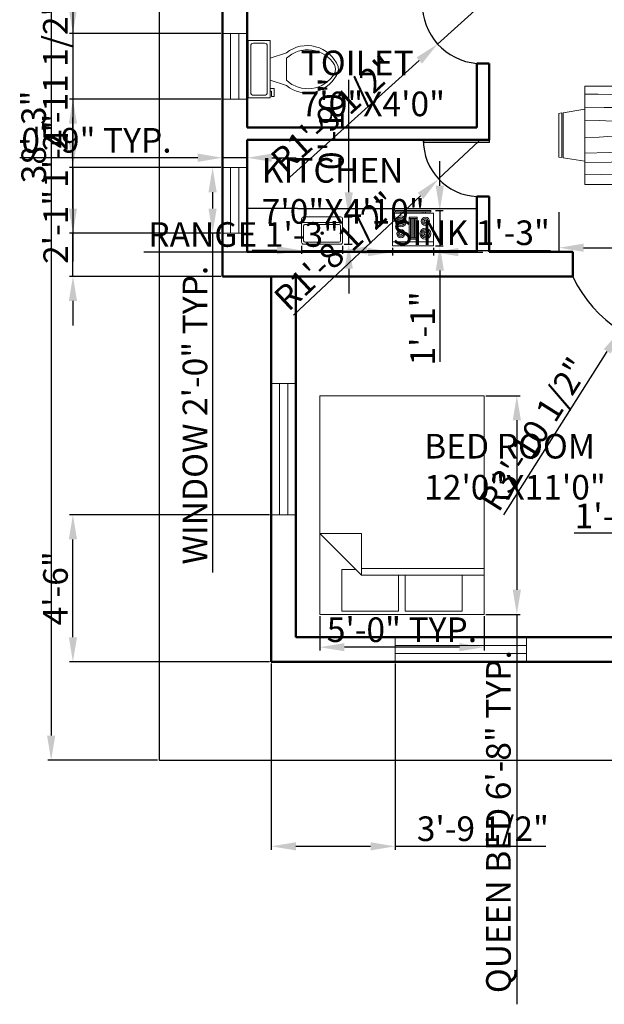
# Model space of a CAD drawing. Units: inches. Extents: x 2059616 to 2060276, y 889994 to 890582.
# Tile 1 of 4: x 2059616 to 2059830, y 889994 to 890354. Entities that reach past the tile are written whole.
import ezdxf

# ---------------------------------------------------------------- set-up
doc = ezdxf.new("R2010")
doc.units = ezdxf.units.IN
for name, color, linetype, lineweight in [('A-ANNO-DIMS', 2, 'Continuous', 18), ('A-AREA-IDEN', 7, 'Continuous', 25), ('A-DOOR', 3, 'Continuous', 25), ('A-EQPM', 9, 'Continuous', 18), ('A-FLOR-CASE', 9, 'Continuous', 25), ('A-FLOR-FIXT', 9, 'Continuous', 18), ('A-FURN', 8, 'Continuous', 18), ('A-GLAZ', 4, 'Continuous', 18), ('A-WALL', 7, 'Continuous', 50), ('C-PROP', 7, 'Continuous', 25)]:
    doc.layers.add(name, color=color, linetype=linetype, lineweight=lineweight)
doc.styles.get("Standard").update_dxf_attribs({"font": 'arial.ttf'})
doc.dimstyles.new('ISO-25', dxfattribs={"dimtxt": 9, "dimasz": 9, "dimexe": 1.25, "dimexo": 0.625, "dimtad": 1, "dimdec": 1, "dimrnd": 9, "dimlunit": 3, "dimtxsty": 'Standard', "dimcen": 2.5, "dimadec": 0, "dimazin": 0, "dimtfac": 1, "dimtdec": 1, "dimtmove": 0, "dimatfit": 3, "dimfxl": 1, "dimarcsym": 0})

# ---------------------------------------------------------------- blocks, each defined once
blk = doc.blocks.new('*D2')
at = {"layer": 'A-ANNO-DIMS', "color": 0, "lineweight": -2, "transparency": 16777216}
for p, q in [((2059666.14, 890538.85), (2059626.05, 890538.85)), ((2059627.3, 890529.85), (2059627.3, 890091.85)), ((2059666.14, 890082.85), (2059626.05, 890082.85))]:
    blk.add_line(p, q, dxfattribs=at)
at = {"layer": 'A-ANNO-DIMS', "color": 0, "transparency": 16777216}
for points in [[(2059625.8, 890529.85), (2059628.8, 890529.85), (2059627.3, 890538.85)], [(2059625.8, 890091.85), (2059628.8, 890091.85), (2059627.3, 890082.85)]]:
    blk.add_solid(points, dxfattribs=at)
at = {"layer": 'Defpoints', "color": 0, "transparency": 16777216}
for p in [(2059666.76, 890538.85), (2059627.3, 890082.85), (2059666.76, 890082.85)]:
    blk.add_point(p, dxfattribs=at)
at = {"layer": 'A-ANNO-DIMS', "color": 0, "transparency": 16777216, "insert": (2059622.08, 890310.85), "char_height": 9, "attachment_point": 5, "rotation": 90}
blk.add_mtext('38\'-3"', dxfattribs=at)
blk = doc.blocks.new('Bed - Queen')
for p, q in [((0, -80.00003), (0, 0)), ((0, 0), (59.99999, 0)), ((59.99999, 0), (59.99999, -80.00003)), ((7.99999, -1.2), (28.79998, -1.2)), ((7.99999, -14.4), (7.99999, -1.2)), ((28.79998, -1.2), (28.79998, -14.4)), ((31.19999, -1.2), (51.99999, -1.2)), ((31.19999, -14.4), (31.19999, -1.2)), ((51.99999, -1.2), (51.99999, -16.4)), ((0, -14.4), (44.8, -14.4)), ((59.99999, -29.6), (44.8, -14.4)), ((44.8, -14.4), (44.8, -29.6)), ((44.8, -16.8), (0, -16.8)), ((51.99999, -16.4), (46.79936, -16.4)), ((44.8, -29.6), (59.99999, -29.6)), ((59.99999, -80.00003), (0, -80.00003))]:
    blk.add_line(p, q)
blk = doc.blocks.new('Toilet - top')
for p, q in [((9.5, -6), (9.5, -2)), ((-10, -8.5), (-8, -8.5)), ((-10, -9.5), (-10, -8.5)), ((-7, -9.5), (-10, -9.5)), ((-8, -8.5), (-8, -8)), ((-7, -8), (-7, -9.5)), ((-4, -8), (-6, -14)), ((4, -8), (6, -14)), ((4, -14), (-4, -14))]:
    blk.add_line(p, q)
blk.add_lwpolyline([(10.5, -8), (10.5, 0), (-10.5, 0), (-10.5, -8)], close=True)
for points in [[(-9.5, -2), (-9.5, -6)], [(8.5, -1), (-8.5, -1)], [(-8.5, -7), (8.5, -7)]]:
    blk.add_lwpolyline(points)
for centre, radius, start, end in [((-8.62, -1.88), 0.884, 81.8699, 188.1301), ((8.62, -1.88), 0.884, 351.8699, 98.1301), ((-8.62, -6.12), 0.884, 171.8699, 278.1301), ((8.62, -6.12), 0.884, 261.8699, 8.1301), ((3.52, -21.58), 12.17, 141.4691, 247.9714), ((4.2, -21.82), 11.33, 136.3677, 238.9468), ((-3.52, -21.58), 12.17, 292.0284, 38.5307), ((-4.2, -21.82), 11.33, 301.053, 43.6321), ((0, -27.88), 4, 245.7318, 294.2682), ((0, -29), 4, 254.8605, 285.1395)]:
    blk.add_arc(centre, radius, start, end)
blk = doc.blocks.new('Range-Oven - 30 in top')
for p, q in [((0, -3), (30, -3)), ((12, -6), (18, -6)), ((13, -20), (13, -6)), ((14, -6), (14, -20)), ((15, -20), (15, -6)), ((16, -6), (16, -20)), ((17, -20), (17, -6)), ((18, -20), (12, -20)), ((6, -24), (6, -25)), ((8, -25), (8, -24)), ((22, -25), (22, -24)), ((24, -24), (24, -25))]:
    blk.add_line(p, q)
for points in [[(0, -24), (0, 0), (30, 0), (30, -24)], [(12, -21), (12, -5), (18, -5), (18, -21)], [(2, -26), (2, -25), (28, -25), (28, -26)]]:
    blk.add_lwpolyline(points, close=True)
for centre, radius in [((6, -9), 4), ((6, -9), 3), ((6, -9), 2), ((24, -9), 3), ((24, -9), 2), ((6, -9), 1), ((24, -18), 4), ((24, -9), 1), ((6, -18), 3), ((6, -18), 2), ((6, -18), 1), ((24, -18), 3), ((24, -18), 2), ((24, -18), 1)]:
    blk.add_circle(centre, radius)
blk = doc.blocks.new('Sink-single - 30 in top')
blk.add_line((-15, -3.999996), (15, -3.999996))
for points in [[(-13.5, 0), (13.5, 0)], [(-15, -18.499996), (-15, -1.5)], [(-13.5, -17.499996), (-13.5, -6.499996)], [(-12.5, -5.499996), (12.5, -5.499996)], [(13.5, -6.499996), (13.5, -17.499996)], [(15, -1.5), (15, -18.499996)], [(13.5, -19.999996), (-13.5, -19.999996)], [(12.5, -18.499996), (-12.5, -18.499996)]]:
    blk.add_lwpolyline(points)
for radius in [1, 0.5]:
    blk.add_circle((0, -11.999996), radius)
for centre, radius, start, end in [((-13.5, -1.5), 1.5, 90, 180), ((-12.5, -6.499996), 1, 90, 180), ((12.5, -6.499996), 1, 0, 90), ((13.5, -1.5), 1.5, 0, 90), ((-13.5, -18.499996), 1.5, 180, 270), ((-12.5, -17.499996), 1, 180, 270), ((12.5, -17.499996), 1, 270, 0), ((13.5, -18.499996), 1.5, 270, 0)]:
    blk.add_arc(centre, radius, start, end)
blk = doc.blocks.new('Dining Set - 36 x 72 in.')
for p, q in [((-22.2343, 26.00059), (-23.4847, 17.99762)), ((-22.2304, 26), (-5.7608, 26)), ((-22, 27.5), (-22.1562, 26.50042)), ((-5.8416, 26.5), (-22.1534, 26.5)), ((-22, 27.5), (-6, 27.5)), ((-5.8437, 26.49966), (-6, 27.5)), ((-4.5152, 17.99762), (-5.7655, 25.99926)), ((5.7657, 26.00059), (4.5153, 17.99762)), ((5.7696, 26), (22.2392, 26)), ((6, 27.5), (5.8438, 26.50042)), ((22.1584, 26.5), (5.8466, 26.5)), ((6, 27.5), (22, 27.5)), ((22.1563, 26.49966), (22, 27.5)), ((23.4848, 17.99762), (22.2345, 25.99926)), ((36, 18), (-36, 18)), ((-36, 18), (-36, -18)), ((36, -18), (36, 18)), ((-45.5, 8), (-44.5004, 8.15617)), ((-45.5, 8), (-45.5, -8)), ((-44.5, -8.15843), (-44.5, 8.15338)), ((-44.0006, 8.23428), (-35.9976, 9.48474)), ((-44, 8.23041), (-44, -8.23915)), ((44.0006, 8.23428), (35.9976, 9.48474)), ((44, 8.23041), (44, -8.23915)), ((44.5, -8.15843), (44.5, 8.15338)), ((45.5, 8), (44.5005, 8.15617)), ((45.5, 8), (45.5, -8)), ((-44.4997, -8.15631), (-45.5, -8)), ((-35.9976, -9.48476), (-43.9993, -8.2345)), ((35.9976, -9.48476), (43.9993, -8.2345)), ((44.4997, -8.15631), (45.5, -8)), ((-36, -18), (36, -18)), ((-22.2343, -26.0006), (-23.4847, -17.99762)), ((-4.5152, -17.99762), (-5.7655, -25.99928)), ((5.7657, -26.0006), (4.5153, -17.99762)), ((23.4848, -17.99762), (22.2345, -25.99928)), ((-22.2304, -26), (-5.7608, -26)), ((-22, -27.5), (-22.1562, -26.50044)), ((-5.8416, -26.5), (-22.1534, -26.5)), ((-22, -27.5), (-6, -27.5)), ((-5.8437, -26.49967), (-6, -27.5)), ((5.7696, -26), (22.2392, -26)), ((6, -27.5), (5.8438, -26.50044)), ((22.1584, -26.5), (5.8466, -26.5)), ((6, -27.5), (22, -27.5)), ((22.1563, -26.49967), (22, -27.5))]:
    blk.add_line(p, q)
for points in [[(-36, 15), (-31.1772, 14.97754), (-26.8079, 14.91406), (-22.8538, 14.81543), (-19.276, 14.6875), (-16.0362, 14.53613), (-13.0957, 14.36718), (-10.4159, 14.18652), (-7.9583, 14), (-5.6904, 13.81315), (-3.6035, 13.63021), (-1.6954, 13.45508), (0.0365, 13.29166), (1.5945, 13.14388), (2.9811, 13.01562), (4.1988, 12.9108), (5.25, 12.83333), (6.1393, 12.78613), (6.8802, 12.76823), (7.4883, 12.77767), (7.9792, 12.8125), (8.3685, 12.87077), (8.6719, 12.95052), (8.9049, 13.0498), (9.0833, 13.16666), (9.2205, 13.29899), (9.3216, 13.44401), (9.3895, 13.59879), (9.4271, 13.76041), (9.4373, 13.92594), (9.4232, 14.09245), (9.3875, 14.257), (9.3333, 14.41666), (9.2638, 14.56917), (9.1836, 14.71484), (9.0975, 14.85465), (9.0104, 14.98958), (8.9272, 15.1206), (8.8529, 15.2487), (8.7922, 15.37483), (8.75, 15.5), (8.7305, 15.62467), (8.7344, 15.74739), (8.7617, 15.86621), (8.8125, 15.97916), (8.8867, 16.08431), (8.9844, 16.17968), (9.1055, 16.26334), (9.25, 16.33333), (9.4189, 16.38802), (9.6172, 16.42708), (9.8506, 16.45052), (10.125, 16.45833), (10.4463, 16.45052), (10.8203, 16.42708), (11.2529, 16.38802), (11.75, 16.33333), (12.3184, 16.26318), (12.9694, 16.17838), (13.7151, 16.07991), (14.5677, 15.96875), (15.5395, 15.84586), (16.6426, 15.71224), (17.8893, 15.56884), (19.2917, 15.41666), (20.859, 15.25667), (22.5879, 15.08984), (24.4721, 14.91715), (26.5052, 14.73958), (28.6809, 14.5581), (30.9929, 14.3737), (33.4347, 14.18733), (36, 14)], [(-36, 10), (-28.9766, 10.14274), (-23.1725, 10.20442), (-18.4241, 10.19775), (-14.5677, 10.13541), (-11.4399, 10.03011), (-8.877, 9.89453), (-6.7154, 9.74137), (-4.7917, 9.58333), (-2.9698, 9.43082), (-1.2246, 9.28515), (0.4415, 9.14534), (2.026, 9.01041), (3.5266, 8.87939), (4.9408, 8.7513), (6.266, 8.62516), (7.5, 8.5), (8.6411, 8.37549), (9.6914, 8.2539), (10.6538, 8.13818), (11.5312, 8.03125), (12.3267, 7.93603), (13.043, 7.85547), (13.6831, 7.79248), (14.25, 7.75), (14.7471, 7.7303), (15.1797, 7.73307), (15.5537, 7.75732), (15.875, 7.80208), (16.1494, 7.86637), (16.3828, 7.94922), (16.5811, 8.04964), (16.75, 8.16666), (16.8944, 8.29915), (17.0143, 8.44531), (17.1089, 8.60319), (17.1771, 8.77083), (17.218, 8.94629), (17.2305, 9.1276), (17.2137, 9.31282), (17.1667, 9.5), (17.0895, 9.6875), (16.987, 9.875), (16.8649, 10.0625), (16.7292, 10.25), (16.5856, 10.4375), (16.4401, 10.625), (16.2985, 10.8125), (16.1667, 11), (16.05, 11.18733), (15.9518, 11.3737), (15.8752, 11.5581), (15.8229, 11.73958), (15.798, 11.91715), (15.8034, 12.08984), (15.842, 12.25667), (15.9167, 12.41666), (16.0295, 12.56836), (16.1784, 12.70833), (16.3605, 12.83268), (16.5729, 12.9375), (16.8127, 13.01888), (17.0768, 13.07291), (17.3625, 13.0957), (17.6667, 13.08333), (17.9894, 13.03312), (18.3418, 12.94726), (18.7382, 12.82918), (19.1927, 12.68229), (19.7195, 12.51001), (20.3327, 12.31575), (21.0465, 12.10294), (21.875, 11.875), (22.8357, 11.63354), (23.959, 11.37304), (25.2786, 11.08618), (26.8282, 10.76562), (28.6414, 10.40405), (30.752, 9.99414), (33.1936, 9.52856), (36, 9)], [(-36, 5.5), (-30.7157, 5.3348), (-26.069, 5.20963), (-21.9946, 5.11767), (-18.4271, 5.05208), (-15.3009, 5.00602), (-12.5508, 4.97265), (-10.1112, 4.94515), (-7.9167, 4.91666), (-5.909, 4.88167), (-4.0586, 4.83984), (-2.3429, 4.79215), (-0.7396, 4.73958), (0.7739, 4.6831), (2.22, 4.6237), (3.6213, 4.56233), (5, 4.5), (6.373, 4.43782), (7.7344, 4.3776), (9.0723, 4.32129), (10.375, 4.27083), (11.6309, 4.22819), (12.8281, 4.19531), (13.9551, 4.17415), (15, 4.16666), (15.954, 4.17448), (16.819, 4.19791), (17.6001, 4.23698), (18.3021, 4.29166), (18.9299, 4.36198), (19.4883, 4.44791), (19.9823, 4.54948), (20.4167, 4.66666), (20.7969, 4.79899), (21.1302, 4.94401), (21.4245, 5.09879), (21.6875, 5.26041), (21.9271, 5.42594), (22.1511, 5.59245), (22.3672, 5.757), (22.5834, 5.91666), (22.8065, 6.06868), (23.0404, 6.21093), (23.2879, 6.34147), (23.5521, 6.45833), (23.8358, 6.55957), (24.142, 6.64323), (24.4735, 6.70735), (24.8334, 6.75), (25.2235, 6.76969), (25.642, 6.76692), (26.0858, 6.74267), (26.5521, 6.69791), (27.0379, 6.63362), (27.5404, 6.55078), (28.0565, 6.45036), (28.5834, 6.33333), (29.1242, 6.19987), (29.7071, 6.04687), (30.3661, 5.87044), (31.1354, 5.66666), (32.0493, 5.43164), (33.142, 5.16146), (34.4475, 4.85221), (36, 4.5)], [(-36, -1), (-30.7915, -0.6591), (-26.0195, -0.38216), (-21.6519, -0.16284), (-17.6563, 0.00521), (-14.0005, 0.12833), (-10.6523, 0.21289), (-7.5796, 0.26522), (-4.75, 0.29166), (-2.134, 0.29793), (0.2878, 0.28711), (2.5317, 0.26163), (4.6146, 0.22396), (6.5529, 0.17651), (8.3633, 0.12174), (10.0623, 0.06209), (11.6667, 0), (13.1899, -0.06201), (14.6341, -0.1211), (15.9982, -0.17432), (17.2813, -0.21875), (18.4823, -0.25147), (19.6003, -0.26953), (20.6343, -0.27002), (21.5834, -0.25), (22.4481, -0.20768), (23.2357, -0.14584), (23.9549, -0.06836), (24.6146, 0.02083), (25.2235, 0.11784), (25.7904, 0.21875), (26.3241, 0.31966), (26.8334, 0.41666), (27.3265, 0.50618), (27.8099, 0.58593), (28.2894, 0.65397), (28.7709, 0.70833), (29.2601, 0.74707), (29.763, 0.76823), (30.2855, 0.76985), (30.8334, 0.75), (31.4088, 0.70784), (31.9994, 0.64713), (32.589, 0.57275), (33.1615, 0.48958), (33.7008, 0.4025), (34.1908, 0.3164), (34.6153, 0.23616), (34.9584, 0.16666), (35.2099, 0.11165), (35.3848, 0.07031), (35.504, 0.04069), (35.5886, 0.02083), (35.6594, 0.00879), (35.7377, 0.0026), (35.8442, 0.00032), (36, 0)], [(-36, -6.5), (-27.1843, -6.31267), (-20.084, -6.1263), (-14.469, -5.9419), (-10.1094, -5.76042), (-6.7752, -5.58285), (-4.2363, -5.41016), (-2.2629, -5.24333), (-0.625, -5.08334), (0.8708, -4.93099), (2.2715, -4.78646), (3.5872, -4.64974), (4.8281, -4.52084), (6.0046, -4.39974), (7.127, -4.28646), (8.2053, -4.18099), (9.25, -4.08334), (10.2705, -3.99382), (11.2734, -3.91407), (12.2647, -3.84603), (13.25, -3.79167), (14.2354, -3.75293), (15.2266, -3.73177), (16.2295, -3.73015), (17.25, -3.75), (18.2912, -3.79248), (19.3451, -3.85547), (20.4009, -3.93604), (21.4479, -4.03125), (22.4754, -4.13819), (23.4727, -4.25391), (24.4289, -4.37549), (25.3334, -4.5), (26.1785, -4.62492), (26.9694, -4.74935), (27.7145, -4.87281), (28.4219, -4.99479), (29.1, -5.11483), (29.7572, -5.23242), (30.4016, -5.34709), (31.0417, -5.45834), (31.6837, -5.56437), (32.3262, -5.65821), (32.9658, -5.73153), (33.599, -5.77604), (34.2224, -5.78345), (34.8327, -5.74545), (35.4264, -5.65373), (36, -5.5)], [(-36, -10), (-26.4022, -9.81299), (-18.4675, -9.62891), (-11.9839, -9.45069), (-6.7396, -9.28125), (-2.5226, -9.12354), (0.8789, -8.98047), (3.6769, -8.85498), (6.0833, -8.75), (8.2767, -8.66765), (10.3021, -8.60677), (12.1712, -8.56543), (13.8958, -8.54167), (15.4876, -8.53353), (16.9583, -8.53907), (18.3197, -8.55632), (19.5834, -8.58334), (20.7616, -8.61841), (21.8685, -8.66081), (22.9188, -8.71004), (23.9271, -8.76563), (24.9081, -8.82707), (25.8763, -8.89388), (26.8465, -8.96558), (27.8334, -9.04167), (28.8474, -9.12118), (29.8828, -9.20117), (30.93, -9.27824), (31.9792, -9.34896), (33.0205, -9.40991), (34.0443, -9.45768), (35.0407, -9.48885), (36, -9.5)], [(-36, -14.5), (-30.0881, -14.33513), (-25.0332, -14.21224), (-20.7312, -14.12647), (-17.0781, -14.07292), (-13.97, -14.04671), (-11.3027, -14.04297), (-8.9724, -14.05681), (-6.875, -14.08334), (-4.9224, -14.11833), (-3.0905, -14.16016), (-1.3709, -14.20785), (0.2448, -14.26042), (1.7647, -14.3169), (3.1973, -14.3763), (4.5507, -14.43767), (5.8333, -14.5), (7.0554, -14.5621), (8.235, -14.62175), (9.3922, -14.67652), (10.5469, -14.72396), (11.7192, -14.76164), (12.929, -14.78711), (14.1965, -14.79794), (15.5417, -14.79167), (16.9933, -14.76424), (18.6152, -14.70508), (20.4804, -14.60197), (22.6615, -14.44271), (25.2312, -14.21509), (28.2624, -13.9069), (31.8277, -13.50594), (36, -13)]]:
    blk.add_lwpolyline(points)
blk = doc.blocks.new('WIN-48IN')
for p, q in [((0, 9), (0, 0)), ((48, 9), (48, 0)), ((48, 6), (0, 6)), ((48, 3), (0, 3))]:
    blk.add_line(p, q)
blk = doc.blocks.new('WIN-24IN')
for p, q in [((0, 24), (9, 24)), ((3, 24), (3, 0)), ((6, 24), (6, 0)), ((0, 0), (9, 0))]:
    blk.add_line(p, q)
blk = doc.blocks.new('*D18')
at = {"layer": 'A-ANNO-DIMS', "color": 0, "lineweight": -2, "transparency": 16777216}
for p, q in [((2059689.29, 890299.64), (2059685.06, 890299.64)), ((2059686.31, 890290.64), (2059686.31, 890284.64)), ((2059689.29, 890275.64), (2059685.06, 890275.64)), ((2059686.31, 890275.64), (2059686.31, 890151.5))]:
    blk.add_line(p, q, dxfattribs=at)
at = {"layer": 'A-ANNO-DIMS', "color": 0, "transparency": 16777216}
for points in [[(2059684.81, 890290.64), (2059687.81, 890290.64), (2059686.31, 890299.64)], [(2059684.81, 890284.64), (2059687.81, 890284.64), (2059686.31, 890275.64)]]:
    blk.add_solid(points, dxfattribs=at)
at = {"layer": 'Defpoints', "color": 0, "transparency": 16777216}
for p in [(2059689.91, 890299.64), (2059686.31, 890275.64), (2059689.91, 890275.64)]:
    blk.add_point(p, dxfattribs=at)
at = {"layer": 'A-ANNO-DIMS', "color": 0, "transparency": 16777216, "insert": (2059681.03, 890209.07), "char_height": 9, "attachment_point": 5, "rotation": 90}
blk.add_mtext('WINDOW 2\'-0" TYP.', dxfattribs=at)
blk = doc.blocks.new('*D19')
at = {"layer": 'A-ANNO-DIMS', "color": 0, "lineweight": -2, "transparency": 16777216}
for p, q in [((2059680.91, 890303.24), (2059615.81, 890303.24)), ((2059689.91, 890300.26), (2059689.91, 890304.49)), ((2059698.91, 890303.24), (2059689.91, 890303.24)), ((2059698.91, 890300.26), (2059698.91, 890304.49)), ((2059707.91, 890303.24), (2059716.91, 890303.24))]:
    blk.add_line(p, q, dxfattribs=at)
at = {"layer": 'A-ANNO-DIMS', "color": 0, "transparency": 16777216}
for points in [[(2059680.91, 890304.74), (2059680.91, 890301.74), (2059689.91, 890303.24)], [(2059707.91, 890304.74), (2059707.91, 890301.74), (2059698.91, 890303.24)]]:
    blk.add_solid(points, dxfattribs=at)
at = {"layer": 'Defpoints', "color": 0, "transparency": 16777216}
for p in [(2059689.91, 890303.24), (2059689.91, 890299.64), (2059698.91, 890299.64)]:
    blk.add_point(p, dxfattribs=at)
at = {"layer": 'A-ANNO-DIMS', "color": 0, "transparency": 16777216, "insert": (2059643.86, 890308.46), "char_height": 9, "attachment_point": 5}
blk.add_mtext('0\'-9" TYP.', dxfattribs=at)
blk = doc.blocks.new('*D22')
at = {"layer": 'A-ANNO-DIMS', "color": 0, "lineweight": -2, "transparency": 16777216}
for p, q in [((2059786.15, 890216.2), (2059798.78, 890216.2)), ((2059797.53, 890207.2), (2059797.53, 890145.2)), ((2059786.15, 890136.2), (2059798.78, 890136.2)), ((2059797.53, 890136.2), (2059797.53, 889993.56))]:
    blk.add_line(p, q, dxfattribs=at)
at = {"layer": 'A-ANNO-DIMS', "color": 0, "transparency": 16777216}
for points in [[(2059796.03, 890207.2), (2059799.03, 890207.2), (2059797.53, 890216.2)], [(2059796.03, 890145.2), (2059799.03, 890145.2), (2059797.53, 890136.2)]]:
    blk.add_solid(points, dxfattribs=at)
at = {"layer": 'Defpoints', "color": 0, "transparency": 16777216}
for p in [(2059785.53, 890216.2), (2059785.53, 890136.2), (2059797.53, 890136.2)]:
    blk.add_point(p, dxfattribs=at)
at = {"layer": 'A-ANNO-DIMS', "color": 0, "transparency": 16777216, "insert": (2059791.97, 890060.38), "char_height": 9, "attachment_point": 5, "rotation": 90}
blk.add_mtext('QUEEN BED 6\'-8" TYP.', dxfattribs=at)
blk = doc.blocks.new('*D23')
at = {"layer": 'A-ANNO-DIMS', "color": 0, "lineweight": -2, "transparency": 16777216}
for p, q in [((2059725.53, 890135.58), (2059725.53, 890122.95)), ((2059785.53, 890135.58), (2059785.53, 890122.95)), ((2059776.53, 890124.2), (2059734.53, 890124.2))]:
    blk.add_line(p, q, dxfattribs=at)
at = {"layer": 'A-ANNO-DIMS', "color": 0, "transparency": 16777216}
for points in [[(2059734.53, 890125.7), (2059734.53, 890122.7), (2059725.53, 890124.2)], [(2059776.53, 890125.7), (2059776.53, 890122.7), (2059785.53, 890124.2)]]:
    blk.add_solid(points, dxfattribs=at)
at = {"layer": 'Defpoints', "color": 0, "transparency": 16777216}
for p in [(2059725.53, 890136.2), (2059785.53, 890136.2), (2059725.53, 890124.2)]:
    blk.add_point(p, dxfattribs=at)
at = {"layer": 'A-ANNO-DIMS', "color": 0, "transparency": 16777216, "insert": (2059755.53, 890129.42), "char_height": 9, "attachment_point": 5}
blk.add_mtext('5\'-0" TYP.', dxfattribs=at)
blk = doc.blocks.new('*D25')
at = {"layer": 'A-ANNO-DIMS', "color": 0, "lineweight": -2, "transparency": 16777216}
for p, q in [((2059882.76, 890161.52), (2059882.76, 890167.1)), ((2059903.76, 890161.52), (2059903.76, 890167.1)), ((2059882.76, 890165.85), (2059818.5, 890165.85)), ((2059894.76, 890165.85), (2059891.76, 890165.85))]:
    blk.add_line(p, q, dxfattribs=at)
at = {"layer": 'A-ANNO-DIMS', "color": 0, "transparency": 16777216}
for points in [[(2059891.76, 890167.35), (2059891.76, 890164.35), (2059882.76, 890165.85)], [(2059894.76, 890167.35), (2059894.76, 890164.35), (2059903.76, 890165.85)]]:
    blk.add_solid(points, dxfattribs=at)
at = {"layer": 'Defpoints', "color": 0, "transparency": 16777216}
for p in [(2059882.76, 890165.85), (2059882.76, 890160.89), (2059903.76, 890160.89)]:
    blk.add_point(p, dxfattribs=at)
at = {"layer": 'A-ANNO-DIMS', "color": 0, "transparency": 16777216, "insert": (2059846.13, 890171.07), "char_height": 9, "attachment_point": 5}
blk.add_mtext('1\'-9" TYP.', dxfattribs=at)
blk = doc.blocks.new('*D32')
at = {"layer": 'A-ANNO-DIMS', "color": 0, "lineweight": -2, "transparency": 16777216}
for p, q in [((2059752.12, 890270.34), (2059752.12, 890267.47)), ((2059767.12, 890270.34), (2059767.12, 890267.47)), ((2059743.12, 890268.72), (2059661.21, 890268.72)), ((2059767.12, 890268.72), (2059752.12, 890268.72)), ((2059776.12, 890268.72), (2059785.12, 890268.72))]:
    blk.add_line(p, q, dxfattribs=at)
at = {"layer": 'A-ANNO-DIMS', "color": 0, "transparency": 16777216}
for points in [[(2059743.12, 890270.22), (2059743.12, 890267.22), (2059752.12, 890268.72)], [(2059776.12, 890270.22), (2059776.12, 890267.22), (2059767.12, 890268.72)]]:
    blk.add_solid(points, dxfattribs=at)
at = {"layer": 'Defpoints', "color": 0, "transparency": 16777216}
for p in [(2059752.12, 890270.97), (2059767.12, 890270.97), (2059752.12, 890268.72)]:
    blk.add_point(p, dxfattribs=at)
at = {"layer": 'A-ANNO-DIMS', "color": 0, "transparency": 16777216, "insert": (2059697.67, 890274), "char_height": 9, "attachment_point": 5}
blk.add_mtext('RANGE 1\'-3"', dxfattribs=at)
blk = doc.blocks.new('*D33')
at = {"layer": 'A-ANNO-DIMS', "color": 0, "lineweight": -2, "transparency": 16777216}
for p, q in [((2059769.37, 890292.97), (2059769.37, 890301.97)), ((2059767.75, 890283.97), (2059770.62, 890283.97)), ((2059769.37, 890283.97), (2059769.37, 890270.97)), ((2059767.75, 890270.97), (2059770.62, 890270.97)), ((2059769.37, 890261.97), (2059769.37, 890228.64))]:
    blk.add_line(p, q, dxfattribs=at)
at = {"layer": 'A-ANNO-DIMS', "color": 0, "transparency": 16777216}
for points in [[(2059767.87, 890292.97), (2059770.87, 890292.97), (2059769.37, 890283.97)], [(2059767.87, 890261.97), (2059770.87, 890261.97), (2059769.37, 890270.97)]]:
    blk.add_solid(points, dxfattribs=at)
at = {"layer": 'Defpoints', "color": 0, "transparency": 16777216}
for p in [(2059767.12, 890283.97), (2059767.12, 890270.97), (2059769.37, 890270.97)]:
    blk.add_point(p, dxfattribs=at)
at = {"layer": 'A-ANNO-DIMS', "color": 0, "transparency": 16777216, "insert": (2059764.23, 890240.8), "char_height": 9, "attachment_point": 5, "rotation": 90}
blk.add_mtext('1\'-1"', dxfattribs=at)
blk = doc.blocks.new('*D34')
at = {"layer": 'A-ANNO-DIMS', "color": 0, "lineweight": -2, "transparency": 16777216}
for p, q in [((2059718.84, 890270.99), (2059718.84, 890268.11)), ((2059733.84, 890270.99), (2059733.84, 890268.11)), ((2059709.84, 890269.36), (2059700.84, 890269.36)), ((2059718.84, 890269.36), (2059733.84, 890269.36)), ((2059742.84, 890269.36), (2059809.81, 890269.36))]:
    blk.add_line(p, q, dxfattribs=at)
at = {"layer": 'A-ANNO-DIMS', "color": 0, "transparency": 16777216}
for points in [[(2059709.84, 890270.86), (2059709.84, 890267.86), (2059718.84, 890269.36)], [(2059742.84, 890270.86), (2059742.84, 890267.86), (2059733.84, 890269.36)]]:
    blk.add_solid(points, dxfattribs=at)
at = {"layer": 'Defpoints', "color": 0, "transparency": 16777216}
for p in [(2059718.84, 890271.61), (2059733.84, 890271.61), (2059733.84, 890269.36)]:
    blk.add_point(p, dxfattribs=at)
at = {"layer": 'A-ANNO-DIMS', "color": 0, "transparency": 16777216, "insert": (2059780.82, 890274.64), "char_height": 9, "attachment_point": 5}
blk.add_mtext('SINK 1\'-3"', dxfattribs=at)
blk = doc.blocks.new('*D35')
at = {"layer": 'A-ANNO-DIMS', "color": 0, "lineweight": -2, "transparency": 16777216}
for p, q in [((2059736.09, 890290.61), (2059736.09, 890331.78)), ((2059734.46, 890281.61), (2059737.34, 890281.61)), ((2059736.09, 890271.61), (2059736.09, 890281.61)), ((2059734.46, 890271.61), (2059737.34, 890271.61)), ((2059736.09, 890262.61), (2059736.09, 890253.61))]:
    blk.add_line(p, q, dxfattribs=at)
at = {"layer": 'A-ANNO-DIMS', "color": 0, "transparency": 16777216}
for points in [[(2059734.59, 890290.61), (2059737.59, 890290.61), (2059736.09, 890281.61)], [(2059734.59, 890262.61), (2059737.59, 890262.61), (2059736.09, 890271.61)]]:
    blk.add_solid(points, dxfattribs=at)
at = {"layer": 'Defpoints', "color": 0, "transparency": 16777216}
for p in [(2059733.84, 890281.61), (2059736.09, 890281.61), (2059733.84, 890271.61)]:
    blk.add_point(p, dxfattribs=at)
at = {"layer": 'A-ANNO-DIMS', "color": 0, "transparency": 16777216, "insert": (2059730.87, 890315.7), "char_height": 9, "attachment_point": 5, "rotation": 90}
blk.add_mtext('0\'-10"', dxfattribs=at)
blk = doc.blocks.new('*D36')
at = {"layer": 'A-ANNO-DIMS', "color": 0, "lineweight": -2, "transparency": 16777216}
for p, q in [((2059812.93, 890283.34), (2059812.93, 890269.07)), ((2059903.93, 890283.34), (2059903.93, 890269.07)), ((2059821.93, 890270.32), (2059894.93, 890270.32)), ((2059903.93, 890270.32), (2060013.1, 890270.32))]:
    blk.add_line(p, q, dxfattribs=at)
at = {"layer": 'A-ANNO-DIMS', "color": 0, "transparency": 16777216}
for points in [[(2059821.93, 890271.82), (2059821.93, 890268.82), (2059812.93, 890270.32)], [(2059894.93, 890271.82), (2059894.93, 890268.82), (2059903.93, 890270.32)]]:
    blk.add_solid(points, dxfattribs=at)
at = {"layer": 'Defpoints', "color": 0, "transparency": 16777216}
for p in [(2059812.93, 890283.97), (2059903.93, 890283.97), (2059903.93, 890270.32)]:
    blk.add_point(p, dxfattribs=at)
at = {"layer": 'A-ANNO-DIMS', "color": 0, "transparency": 16777216, "insert": (2059963.02, 890275.59), "char_height": 9, "attachment_point": 5}
blk.add_mtext('DINING SET 7\'-7"', dxfattribs=at)
blk = doc.blocks.new('*D40')
at = {"layer": 'A-ANNO-DIMS', "color": 0, "lineweight": -2, "transparency": 16777216}
for p, q in [((2059707.14, 890404.26), (2059634.01, 890404.26)), ((2059635.26, 890395.26), (2059635.26, 890377.85)), ((2059707.14, 890368.85), (2059634.01, 890368.85)), ((2059635.26, 890368.85), (2059635.26, 890306.55))]:
    blk.add_line(p, q, dxfattribs=at)
at = {"layer": 'A-ANNO-DIMS', "color": 0, "transparency": 16777216}
for points in [[(2059633.76, 890395.26), (2059636.76, 890395.26), (2059635.26, 890404.26)], [(2059633.76, 890377.85), (2059636.76, 890377.85), (2059635.26, 890368.85)]]:
    blk.add_solid(points, dxfattribs=at)
at = {"layer": 'Defpoints', "color": 0, "transparency": 16777216}
for p in [(2059707.76, 890404.26), (2059635.26, 890368.85), (2059707.76, 890368.85)]:
    blk.add_point(p, dxfattribs=at)
at = {"layer": 'A-ANNO-DIMS', "color": 0, "transparency": 16777216, "insert": (2059629.98, 890333.2), "char_height": 9, "attachment_point": 5, "rotation": 90}
blk.add_mtext('2\'-11 1/2"', dxfattribs=at)
blk = doc.blocks.new('*D41')
at = {"layer": 'A-ANNO-DIMS', "color": 0, "lineweight": -2, "transparency": 16777216}
for p, q in [((2059689.29, 890324.68), (2059634.01, 890324.68)), ((2059635.26, 890315.68), (2059635.26, 890308.64)), ((2059689.29, 890299.64), (2059634.01, 890299.64)), ((2059635.26, 890299.64), (2059635.26, 890265.31))]:
    blk.add_line(p, q, dxfattribs=at)
at = {"layer": 'A-ANNO-DIMS', "color": 0, "transparency": 16777216}
for points in [[(2059633.76, 890315.68), (2059636.76, 890315.68), (2059635.26, 890324.68)], [(2059633.76, 890308.64), (2059636.76, 890308.64), (2059635.26, 890299.64)]]:
    blk.add_solid(points, dxfattribs=at)
at = {"layer": 'Defpoints', "color": 0, "transparency": 16777216}
for p in [(2059689.91, 890324.68), (2059635.26, 890299.64), (2059689.91, 890299.64)]:
    blk.add_point(p, dxfattribs=at)
at = {"layer": 'A-ANNO-DIMS', "color": 0, "transparency": 16777216, "insert": (2059630.12, 890277.97), "char_height": 9, "attachment_point": 5, "rotation": 90}
blk.add_mtext('2\'-1"', dxfattribs=at)
blk = doc.blocks.new('*D48')
at = {"layer": 'A-ANNO-DIMS', "color": 0, "lineweight": -2, "transparency": 16777216}
for p, q in [((2059707.14, 890172.64), (2059634.01, 890172.64)), ((2059635.26, 890127.85), (2059635.26, 890163.64)), ((2059707.14, 890118.85), (2059634.01, 890118.85))]:
    blk.add_line(p, q, dxfattribs=at)
at = {"layer": 'A-ANNO-DIMS', "color": 0, "transparency": 16777216}
for points in [[(2059633.76, 890163.64), (2059636.76, 890163.64), (2059635.26, 890172.64)], [(2059633.76, 890127.85), (2059636.76, 890127.85), (2059635.26, 890118.85)]]:
    blk.add_solid(points, dxfattribs=at)
at = {"layer": 'Defpoints', "color": 0, "transparency": 16777216}
for p in [(2059635.26, 890172.64), (2059707.76, 890172.64), (2059707.76, 890118.85)]:
    blk.add_point(p, dxfattribs=at)
at = {"layer": 'A-ANNO-DIMS', "color": 0, "transparency": 16777216, "insert": (2059630.04, 890145.74), "char_height": 9, "attachment_point": 5, "rotation": 90}
blk.add_mtext('4\'-6"', dxfattribs=at)
blk = doc.blocks.new('*D49')
at = {"layer": 'A-ANNO-DIMS', "color": 0, "lineweight": -2, "transparency": 16777216}
for p, q in [((2059635.26, 890368.85), (2059635.26, 890402.17)), ((2059689.29, 890368.85), (2059634.01, 890368.85)), ((2059635.26, 890357.68), (2059635.26, 890359.85)), ((2059689.29, 890348.68), (2059634.01, 890348.68))]:
    blk.add_line(p, q, dxfattribs=at)
at = {"layer": 'A-ANNO-DIMS', "color": 0, "transparency": 16777216}
for points in [[(2059633.76, 890359.85), (2059636.76, 890359.85), (2059635.26, 890368.85)], [(2059633.76, 890357.68), (2059636.76, 890357.68), (2059635.26, 890348.68)]]:
    blk.add_solid(points, dxfattribs=at)
at = {"layer": 'Defpoints', "color": 0, "transparency": 16777216}
for p in [(2059635.26, 890368.85), (2059689.91, 890368.85), (2059689.91, 890348.68)]:
    blk.add_point(p, dxfattribs=at)
at = {"layer": 'A-ANNO-DIMS', "color": 0, "transparency": 16777216, "insert": (2059630.04, 890390.01), "char_height": 9, "attachment_point": 5, "rotation": 90}
blk.add_mtext('1\'-8"', dxfattribs=at)
blk = doc.blocks.new('*D50')
at = {"layer": 'A-ANNO-DIMS', "color": 0, "lineweight": -2, "transparency": 16777216}
for p, q in [((2059635.26, 890284.64), (2059635.26, 890317.96)), ((2059689.29, 890275.64), (2059634.01, 890275.64)), ((2059635.26, 890259.85), (2059635.26, 890275.64)), ((2059689.29, 890259.85), (2059634.01, 890259.85)), ((2059635.26, 890250.85), (2059635.26, 890241.85))]:
    blk.add_line(p, q, dxfattribs=at)
at = {"layer": 'A-ANNO-DIMS', "color": 0, "transparency": 16777216}
for points in [[(2059633.76, 890284.64), (2059636.76, 890284.64), (2059635.26, 890275.64)], [(2059633.76, 890250.85), (2059636.76, 890250.85), (2059635.26, 890259.85)]]:
    blk.add_solid(points, dxfattribs=at)
at = {"layer": 'Defpoints', "color": 0, "transparency": 16777216}
for p in [(2059635.26, 890275.64), (2059689.91, 890275.64), (2059689.91, 890259.85)]:
    blk.add_point(p, dxfattribs=at)
at = {"layer": 'A-ANNO-DIMS', "color": 0, "transparency": 16777216, "insert": (2059630.12, 890305.8), "char_height": 9, "attachment_point": 5, "rotation": 90}
blk.add_mtext('1\'-4"', dxfattribs=at)
blk = doc.blocks.new('*D51')
at = {"layer": 'A-ANNO-DIMS', "color": 0, "lineweight": -2, "transparency": 16777216}
for p, q in [((2059707.76, 890118.22), (2059707.76, 890050.1)), ((2059753.04, 890118.22), (2059753.04, 890050.1)), ((2059716.76, 890051.35), (2059744.04, 890051.35)), ((2059753.04, 890051.35), (2059808.18, 890051.35))]:
    blk.add_line(p, q, dxfattribs=at)
at = {"layer": 'A-ANNO-DIMS', "color": 0, "transparency": 16777216}
for points in [[(2059716.76, 890052.85), (2059716.76, 890049.85), (2059707.76, 890051.35)], [(2059744.04, 890052.85), (2059744.04, 890049.85), (2059753.04, 890051.35)]]:
    blk.add_solid(points, dxfattribs=at)
at = {"layer": 'Defpoints', "color": 0, "transparency": 16777216}
for p in [(2059707.76, 890118.85), (2059753.04, 890118.85), (2059753.04, 890051.35)]:
    blk.add_point(p, dxfattribs=at)
at = {"layer": 'A-ANNO-DIMS', "color": 0, "transparency": 16777216, "insert": (2059785.11, 890056.63), "char_height": 9, "attachment_point": 5}
blk.add_mtext('3\'-9 1/2"', dxfattribs=at)
blk = doc.blocks.new('*D60')
at = {"layer": 'A-ANNO-DIMS', "color": 0, "lineweight": -2, "transparency": 16777216}
for p, q in [((2059860.26, 890279.49), (2059835.38, 890240.04)), ((2059792.83, 890172.58), (2059830.58, 890232.42))]:
    blk.add_line(p, q, dxfattribs=at)
at = {"layer": 'A-ANNO-DIMS', "color": 0, "transparency": 16777216}
blk.add_solid([(2059829.31, 890233.22), (2059831.85, 890231.62), (2059835.38, 890240.04)], dxfattribs=at)
at = {"layer": 'Defpoints', "color": 0, "transparency": 16777216}
for p in [(2059860.26, 890279.49), (2059835.38, 890240.04)]:
    blk.add_point(p, dxfattribs=at)
at = {"layer": 'A-ANNO-DIMS', "color": 0, "transparency": 16777216, "insert": (2059804.84, 890201.51), "char_height": 9, "attachment_point": 5, "rotation": 57.7581}
blk.add_mtext('R3\'-10 1/2"', dxfattribs=at)
blk = doc.blocks.new('*D64')
at = {"layer": 'A-ANNO-DIMS', "color": 0, "lineweight": -2, "transparency": 16777216}
for p, q in [((2059784.66, 890359.35), (2059768.57, 890344.84)), ((2059714.52, 890296.13), (2059761.88, 890338.82))]:
    blk.add_line(p, q, dxfattribs=at)
at = {"layer": 'A-ANNO-DIMS', "color": 0, "transparency": 16777216}
blk.add_solid([(2059760.88, 890339.93), (2059762.89, 890337.7), (2059768.57, 890344.84)], dxfattribs=at)
at = {"layer": 'Defpoints', "color": 0, "transparency": 16777216}
for p in [(2059784.66, 890359.35), (2059768.57, 890344.84)]:
    blk.add_point(p, dxfattribs=at)
at = {"layer": 'A-ANNO-DIMS', "color": 0, "transparency": 16777216, "insert": (2059731.33, 890318.38), "char_height": 9, "attachment_point": 5, "rotation": 42.0332}
blk.add_mtext('R1\'-9 1/2"', dxfattribs=at)
blk = doc.blocks.new('*D65')
at = {"layer": 'A-ANNO-DIMS', "color": 0, "lineweight": -2, "transparency": 16777216}
for p, q in [((2059783.68, 890309.35), (2059768.91, 890295.47)), ((2059715.87, 890245.65), (2059762.35, 890289.3))]:
    blk.add_line(p, q, dxfattribs=at)
at = {"layer": 'A-ANNO-DIMS', "color": 0, "transparency": 16777216}
blk.add_solid([(2059761.32, 890290.4), (2059763.37, 890288.21), (2059768.91, 890295.47)], dxfattribs=at)
at = {"layer": 'Defpoints', "color": 0, "transparency": 16777216}
for p in [(2059783.68, 890309.35), (2059768.91, 890295.47)]:
    blk.add_point(p, dxfattribs=at)
at = {"layer": 'A-ANNO-DIMS', "color": 0, "transparency": 16777216, "insert": (2059732.22, 890268.24), "char_height": 9, "attachment_point": 5, "rotation": 43.2076}
blk.add_mtext('R1\'-8 1/2"', dxfattribs=at)

msp = doc.modelspace()

# ---------------------------------------------------------------- linework, layer by layer
at = {"layer": 'A-DOOR'}
for p, q in [((2059763.41, 890308.85), (2059763.41, 890309.85)), ((2059787.41, 890308.85), (2059763.41, 890308.85)), ((2059787.41, 890309.85), (2059787.41, 890308.85))]:
    msp.add_line(p, q, dxfattribs=at)
for centre, radius, start, end in [((2059784.66, 890359.35), 21.66, 178.6774, 265.3869), ((2059783.68, 890309.35), 20.27, 178.5869, 267.8277), ((2059860.26, 890279.49), 46.64, 204.9024, 270.6142)]:
    msp.add_arc(centre, radius, start, end, dxfattribs=at)
at = {"layer": 'A-FLOR-CASE'}
for q in [(2059698.91, 890284.69), (2059782.91, 890284.69)]:
    msp.add_line((2059717.32, 890284.69), q, dxfattribs=at)
at = {"layer": 'A-WALL'}
for p, q in [((2059689.91, 890359.85), (2059689.91, 890259.85)), ((2059698.91, 890359.85), (2059698.91, 890314.35)), ((2059782.91, 890337.75), (2059782.91, 890314.35)), ((2059782.91, 890337.75), (2059787.41, 890337.75)), ((2059787.41, 890337.75), (2059787.41, 890309.85)), ((2059698.91, 890314.35), (2059782.91, 890314.35)), ((2059698.91, 890309.85), (2059787.41, 890309.85)), ((2059698.91, 890309.85), (2059698.91, 890268.85)), ((2059782.91, 890289.09), (2059787.41, 890289.09)), ((2059782.91, 890289.09), (2059782.91, 890268.85)), ((2059787.41, 890289.09), (2059787.41, 890268.85)), ((2059716.76, 890268.85), (2059698.91, 890268.85)), ((2059716.76, 890268.85), (2059782.91, 890268.85)), ((2059787.41, 890268.85), (2059817.96, 890268.85)), ((2059817.96, 890268.85), (2059817.96, 890259.85)), ((2059689.91, 890259.85), (2059694.15, 890259.85)), ((2059694.15, 890259.85), (2059817.96, 890259.85)), ((2059707.76, 890118.85), (2059707.76, 890259.85)), ((2059716.76, 890127.85), (2059716.76, 890259.85)), ((2059716.76, 890127.85), (2059860.76, 890127.85)), ((2059707.76, 890118.85), (2059925.76, 890118.85))]:
    msp.add_line(p, q, dxfattribs=at)
at = {"layer": 'C-PROP'}
for p, q in [((2059666.76, 890538.85), (2059666.76, 890082.85)), ((2059666.76, 890082.85), (2060242.76, 890082.85))]:
    msp.add_line(p, q, dxfattribs=at)

# ---------------------------------------------------------------- block references
at = {"layer": 'A-EQPM', "xscale": 0.5, "yscale": 0.5, "rotation": 180}
msp.add_blockref('Range-Oven - 30 in top', (2059767.12, 890270.97), dxfattribs=at)
at = {"layer": 'A-FLOR-FIXT', "rotation": 90}
msp.add_blockref('Toilet - top', (2059699.31, 890335.62), dxfattribs=at)
at = {"layer": 'A-FLOR-FIXT', "xscale": 0.5, "yscale": 0.5}
msp.add_blockref('Sink-single - 30 in top', (2059726.34, 890281.61), dxfattribs=at)
at = {"layer": 'A-FURN'}
msp.add_blockref('Dining Set - 36 x 72 in.', (2059858.43, 890311.47), dxfattribs=at)
at = {"layer": 'A-FURN', "rotation": 180}
msp.add_blockref('Bed - Queen', (2059785.53, 890136.2), dxfattribs=at)
at = {"layer": 'A-GLAZ'}
for name, p in [('WIN-24IN', (2059689.92, 890324.68)), ('WIN-48IN', (2059753.04, 890118.85))]:
    msp.add_blockref(name, p, dxfattribs=at)
for name, p, rotation in [('WIN-24IN', (2059698.91, 890299.64), 180), ('WIN-48IN', (2059707.76, 890220.64), 270.0000000000671)]:
    msp.add_blockref(name, p, dxfattribs=dict(at, rotation=rotation))

# ---------------------------------------------------------------- texts
at = {"layer": 'A-AREA-IDEN', "char_height": 9, "attachment_point": 1}
for s, insert in [('TOILET\\P7\'0"X4\'0"', (2059718.52, 890342.44)), ('KITCHEN\\P7\'0"X4\'10"', (2059704.29, 890303.11)), ('BED ROOM\\P12\'0"X11\'0"', (2059763.66, 890202.22))]:
    msp.add_mtext_dynamic_manual_height_columns(s, width=69.4215, gutter_width=12.5, heights=[0], dxfattribs=dict(at, insert=insert))

# ---------------------------------------------------------------- dimensions: what is measured, and where the dimension line sits
at = {"layer": 'A-ANNO-DIMS'}
for base, p1, p2, angle, override, picture, middle in [((2059627.3, 890082.85), (2059666.76, 890538.85), (2059666.76, 890082.85), 90, {"dimclrd": 0, "dimclre": 0, "dimclrt": 0}, '*D2', (2059622.08, 890310.85)), ((2059635.26, 890368.85), (2059707.76, 890404.26), (2059707.76, 890368.85), 90, {"dimdec": 1, "dimlfac": 1, "dimrnd": 0, "dimzin": 1, "dimdsep": 46, "dimlunit": 4, "dimfrac": 2}, '*D40', (2059629.98, 890333.2)), ((2059635.26, 890368.85), (2059689.91, 890348.68), (2059689.91, 890368.85), 90, {"dimdec": 1, "dimlfac": 1, "dimrnd": 0, "dimzin": 1, "dimdsep": 46, "dimlunit": 4, "dimfrac": 2}, '*D49', (2059630.04, 890390.01)), ((2059736.09, 890281.61), (2059733.84, 890271.61), (2059733.84, 890281.61), 90, {"dimdec": 1, "dimlfac": 1, "dimrnd": 0, "dimzin": 1, "dimdsep": 46, "dimlunit": 4, "dimfrac": 2}, '*D35', (2059730.87, 890315.7)), ((2059635.26, 890299.64), (2059689.91, 890324.68), (2059689.91, 890299.64), 90, {"dimdec": 1, "dimlfac": 1, "dimrnd": 0, "dimzin": 1, "dimdsep": 46, "dimlunit": 4, "dimfrac": 2}, '*D41', (2059630.12, 890277.97)), ((2059635.26, 890275.64), (2059689.91, 890259.85), (2059689.91, 890275.64), 90, {"dimdec": 1, "dimlfac": 1, "dimrnd": 0, "dimzin": 1, "dimdsep": 46, "dimlunit": 4, "dimfrac": 2}, '*D50', (2059630.12, 890305.8)), ((2059769.37, 890270.97), (2059767.12, 890283.97), (2059767.12, 890270.97), 270, {"dimdec": 1, "dimlfac": 1, "dimrnd": 0, "dimzin": 1, "dimdsep": 46, "dimlunit": 4, "dimfrac": 2}, '*D33', (2059764.23, 890240.8)), ((2059635.26, 890172.64), (2059707.76, 890118.85), (2059707.76, 890172.64), 90, {"dimdec": 1, "dimlfac": 1, "dimrnd": 0, "dimzin": 1, "dimdsep": 46, "dimlunit": 4, "dimfrac": 2}, '*D48', (2059630.04, 890145.74))]:
    dim = msp.add_linear_dim(base=base, p1=p1, p2=p2, angle=angle, dimstyle='ISO-25', override=override, dxfattribs=at)
    dim.commit()
    dim.dimension.update_dxf_attribs({"geometry": picture, "text_midpoint": middle})
for center, mpoint, picture, middle in [((2059784.66, 890359.35), (2059768.57, 890344.84), '*D64', (2059731.33, 890318.38)), ((2059783.68, 890309.35), (2059768.91, 890295.47), '*D65', (2059732.22, 890268.24)), ((2059860.26, 890279.49), (2059835.38, 890240.04), '*D60', (2059804.84, 890201.51))]:
    dim = msp.add_radius_dim(center=center, mpoint=mpoint, dimstyle='ISO-25', override={"dimdec": 1, "dimlfac": 1, "dimrnd": 0, "dimzin": 1, "dimdsep": 46, "dimlunit": 4, "dimfrac": 2}, dxfattribs=at)
    dim.commit()
    dim.dimension.update_dxf_attribs({"geometry": picture, "text_midpoint": middle})
for base, p1, p2, angle, text, picture, middle in [((2059689.91, 890303.24), (2059698.91, 890299.64), (2059689.91, 890299.64), 180, '<> TYP.', '*D19', (2059643.86, 890308.46)), ((2059686.31, 890275.64), (2059689.91, 890299.64), (2059689.91, 890275.64), 270, 'WINDOW <> TYP.', '*D18', (2059681.03, 890209.07)), ((2059752.12, 890268.72), (2059767.12, 890270.97), (2059752.12, 890270.97), 180, 'RANGE <>', '*D32', (2059697.67, 890274)), ((2059797.53, 890136.2), (2059785.53, 890216.2), (2059785.53, 890136.2), 270, 'QUEEN BED <> TYP.', '*D22', (2059791.97, 890060.38)), ((2059882.76, 890165.85), (2059903.76, 890160.89), (2059882.76, 890160.89), 180, '<> TYP.', '*D25', (2059846.13, 890171.07)), ((2059725.53, 890124.2), (2059785.53, 890136.2), (2059725.53, 890136.2), 180, '<> TYP.', '*D23', (2059755.53, 890129.42))]:
    dim = msp.add_linear_dim(base=base, p1=p1, p2=p2, angle=angle, text=text, dimstyle='ISO-25', override={"dimdec": 1, "dimlfac": 1, "dimrnd": 0, "dimzin": 1, "dimdsep": 46, "dimlunit": 4, "dimfrac": 2}, dxfattribs=at)
    dim.commit()
    dim.dimension.update_dxf_attribs({"geometry": picture, "text_midpoint": middle})
for base, p1, p2, text, picture, middle in [((2059903.93, 890270.32), (2059812.93, 890283.97), (2059903.93, 890283.97), 'DINING SET <>', '*D36', (2059963.02, 890275.59)), ((2059733.84, 890269.36), (2059718.84, 890271.61), (2059733.84, 890271.61), 'SINK <>', '*D34', (2059780.82, 890274.64))]:
    dim = msp.add_linear_dim(base=base, p1=p1, p2=p2, text=text, dimstyle='ISO-25', override={"dimdec": 1, "dimlfac": 1, "dimrnd": 0, "dimzin": 1, "dimdsep": 46, "dimlunit": 4, "dimfrac": 2}, dxfattribs=at)
    dim.commit()
    dim.dimension.update_dxf_attribs({"geometry": picture, "text_midpoint": middle})
dim = msp.add_linear_dim(base=(2059753.04, 890051.35), p1=(2059707.76, 890118.85), p2=(2059753.04, 890118.85), dimstyle='ISO-25', override={"dimdec": 1, "dimlfac": 1, "dimrnd": 0, "dimzin": 1, "dimdsep": 46, "dimlunit": 4, "dimfrac": 2}, dxfattribs=at)
dim.commit()
dim.dimension.update_dxf_attribs({"geometry": '*D51', "text_midpoint": (2059785.11, 890056.63)})

doc.saveas('drawing.dxf')
